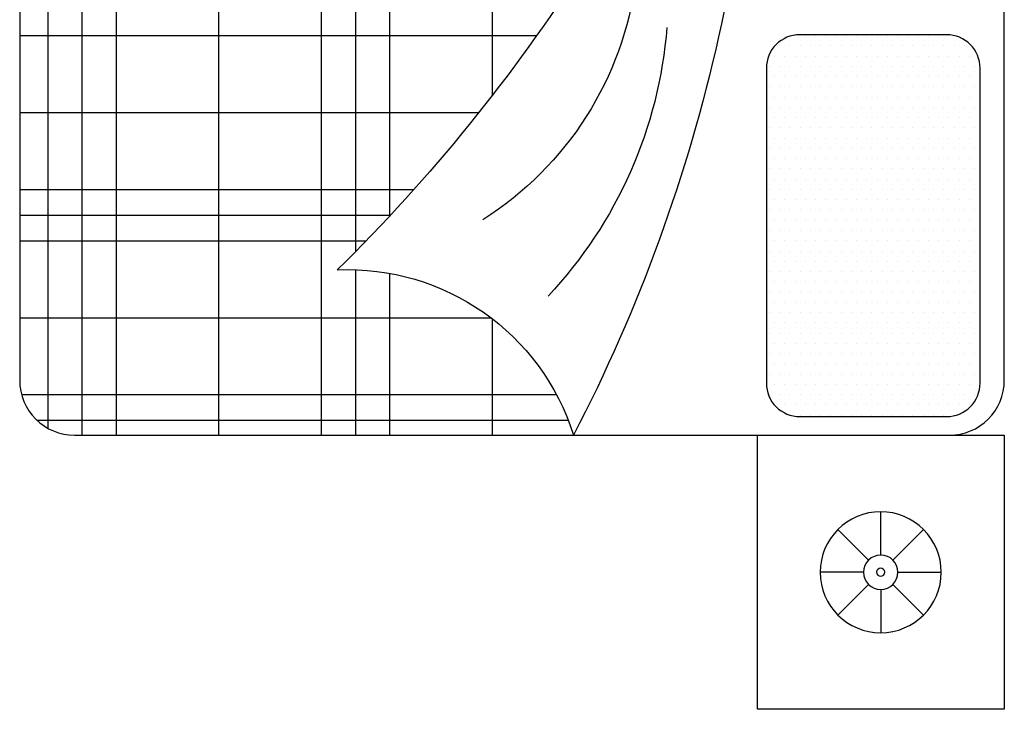
# Model space of a CAD drawing. Units: inches. Extents: x 528 to 2520, y -151 to 1354.
# Tile 11 of 41: x 814 to 869, y 1151 to 1189. Entities that reach past the tile are written whole.
import ezdxf

# ---------------------------------------------------------------- set-up
doc = ezdxf.new("R2010")
doc.units = ezdxf.units.IN
doc.header["$MEASUREMENT"] = 0
doc.layers.add('A-FURN', color=8, linetype='Continuous', lineweight=18)
doc.layers.add('BLOCK', color=6, linetype='Continuous')

# ---------------------------------------------------------------- blocks, each defined once
blk = doc.blocks.new('*X15')
at = {"color": 0}
for p, q in [((276.598, 451.25), (280.51, 451.25)), ((275.455, 450.625), (280.51, 450.625)), ((274.411, 450), (280.51, 450)), ((265.51, 448.125), (267.634, 448.125)), ((271.723, 448.125), (280.51, 448.125)), ((265.51, 446.25), (268.465, 446.25)), ((269.519, 446.25), (280.51, 446.25)), ((265.51, 445.625), (268.531, 445.625)), ((268.866, 445.625), (280.51, 445.625)), ((265.51, 445), (280.51, 445)), ((265.51, 443.125), (280.51, 443.125)), ((265.51, 441.25), (280.51, 441.25)), ((265.51, 440.625), (280.51, 440.625)), ((265.634, 440), (280.386, 440))]:
    blk.add_line(p, q, dxfattribs=at)
blk = doc.blocks.new('*X16')
at = {"color": 0}
for p, q in [((280.312, 439.886), (280.312, 452.896)), ((278.906, 439.482), (278.906, 452.338)), ((277.5, 439.482), (277.5, 451.702)), ((277.031, 439.482), (277.031, 451.471)), ((276.562, 439.482), (276.562, 451.231)), ((275.156, 439.482), (275.156, 450.451)), ((265.781, 439.797), (265.781, 449.511)), ((273.75, 439.482), (273.75, 449.576)), ((266.25, 439.517), (266.25, 449.296)), ((273.281, 439.482), (273.281, 449.261)), ((272.812, 439.482), (272.812, 448.934)), ((267.656, 439.482), (267.656, 448.095)), ((271.406, 439.482), (271.406, 447.876)), ((270, 439.482), (270, 446.689)), ((269.531, 439.482), (269.531, 446.262)), ((269.062, 439.482), (269.062, 445.817))]:
    blk.add_line(p, q, dxfattribs=at)
blk = doc.blocks.new('*X17')
at = {"color": 0}
for p, q in [((266.4375, 457.03125), (266.4375, 457.03125)), ((266.8125, 457.03125), (266.8125, 457.03125)), ((267.1875, 457.03125), (267.1875, 457.03125)), ((267.5625, 457.03125), (267.5625, 457.03125)), ((267.9375, 457.03125), (267.9375, 457.03125)), ((268.3125, 457.03125), (268.3125, 457.03125)), ((268.6875, 457.03125), (268.6875, 457.03125)), ((269.0625, 457.03125), (269.0625, 457.03125)), ((269.4375, 457.03125), (269.4375, 457.03125)), ((269.8125, 457.03125), (269.8125, 457.03125)), ((270.1875, 457.03125), (270.1875, 457.03125)), ((270.5625, 457.03125), (270.5625, 457.03125)), ((270.9375, 457.03125), (270.9375, 457.03125)), ((271.3125, 457.03125), (271.3125, 457.03125)), ((271.6875, 457.03125), (271.6875, 457.03125)), ((272.0625, 457.03125), (272.0625, 457.03125)), ((266.0625, 456.84375), (266.0625, 456.84375)), ((266.25, 456.9375), (266.25, 456.9375)), ((266.4375, 456.84375), (266.4375, 456.84375)), ((266.625, 456.9375), (266.625, 456.9375)), ((266.8125, 456.84375), (266.8125, 456.84375)), ((267, 456.9375), (267, 456.9375)), ((267.1875, 456.84375), (267.1875, 456.84375)), ((267.375, 456.9375), (267.375, 456.9375)), ((267.5625, 456.84375), (267.5625, 456.84375)), ((267.75, 456.9375), (267.75, 456.9375)), ((267.9375, 456.84375), (267.9375, 456.84375)), ((268.125, 456.9375), (268.125, 456.9375)), ((268.3125, 456.84375), (268.3125, 456.84375)), ((268.5, 456.9375), (268.5, 456.9375)), ((268.6875, 456.84375), (268.6875, 456.84375)), ((268.875, 456.9375), (268.875, 456.9375)), ((269.0625, 456.84375), (269.0625, 456.84375)), ((269.25, 456.9375), (269.25, 456.9375)), ((269.4375, 456.84375), (269.4375, 456.84375)), ((269.625, 456.9375), (269.625, 456.9375)), ((269.8125, 456.84375), (269.8125, 456.84375)), ((270, 456.9375), (270, 456.9375)), ((270.1875, 456.84375), (270.1875, 456.84375)), ((270.375, 456.9375), (270.375, 456.9375)), ((270.5625, 456.84375), (270.5625, 456.84375)), ((270.75, 456.9375), (270.75, 456.9375)), ((270.9375, 456.84375), (270.9375, 456.84375)), ((271.125, 456.9375), (271.125, 456.9375)), ((271.3125, 456.84375), (271.3125, 456.84375)), ((271.5, 456.9375), (271.5, 456.9375)), ((271.6875, 456.84375), (271.6875, 456.84375)), ((271.875, 456.9375), (271.875, 456.9375)), ((272.0625, 456.84375), (272.0625, 456.84375)), ((272.25, 456.9375), (272.25, 456.9375)), ((272.4375, 456.84375), (272.4375, 456.84375)), ((266.25, 456.75), (266.25, 456.75)), ((266.625, 456.75), (266.625, 456.75)), ((267, 456.75), (267, 456.75)), ((267.375, 456.75), (267.375, 456.75)), ((267.75, 456.75), (267.75, 456.75)), ((268.125, 456.75), (268.125, 456.75)), ((268.5, 456.75), (268.5, 456.75)), ((268.875, 456.75), (268.875, 456.75)), ((269.25, 456.75), (269.25, 456.75)), ((269.625, 456.75), (269.625, 456.75)), ((270, 456.75), (270, 456.75)), ((270.375, 456.75), (270.375, 456.75)), ((270.75, 456.75), (270.75, 456.75)), ((271.125, 456.75), (271.125, 456.75)), ((271.5, 456.75), (271.5, 456.75)), ((271.875, 456.75), (271.875, 456.75)), ((272.25, 456.75), (272.25, 456.75)), ((272.625, 456.75), (272.625, 456.75)), ((265.875, 456.5625), (265.875, 456.5625)), ((266.0625, 456.65625), (266.0625, 456.65625)), ((266.25, 456.5625), (266.25, 456.5625)), ((266.4375, 456.65625), (266.4375, 456.65625)), ((266.625, 456.5625), (266.625, 456.5625)), ((266.8125, 456.65625), (266.8125, 456.65625)), ((267, 456.5625), (267, 456.5625)), ((267.1875, 456.65625), (267.1875, 456.65625)), ((267.375, 456.5625), (267.375, 456.5625)), ((267.5625, 456.65625), (267.5625, 456.65625)), ((267.75, 456.5625), (267.75, 456.5625)), ((267.9375, 456.65625), (267.9375, 456.65625)), ((268.125, 456.5625), (268.125, 456.5625)), ((268.3125, 456.65625), (268.3125, 456.65625)), ((268.5, 456.5625), (268.5, 456.5625)), ((268.6875, 456.65625), (268.6875, 456.65625)), ((268.875, 456.5625), (268.875, 456.5625)), ((269.0625, 456.65625), (269.0625, 456.65625)), ((269.25, 456.5625), (269.25, 456.5625)), ((269.4375, 456.65625), (269.4375, 456.65625)), ((269.625, 456.5625), (269.625, 456.5625)), ((269.8125, 456.65625), (269.8125, 456.65625)), ((270, 456.5625), (270, 456.5625)), ((270.1875, 456.65625), (270.1875, 456.65625)), ((270.375, 456.5625), (270.375, 456.5625)), ((270.5625, 456.65625), (270.5625, 456.65625)), ((270.75, 456.5625), (270.75, 456.5625)), ((270.9375, 456.65625), (270.9375, 456.65625)), ((271.125, 456.5625), (271.125, 456.5625)), ((271.3125, 456.65625), (271.3125, 456.65625)), ((271.5, 456.5625), (271.5, 456.5625)), ((271.6875, 456.65625), (271.6875, 456.65625)), ((271.875, 456.5625), (271.875, 456.5625)), ((272.0625, 456.65625), (272.0625, 456.65625)), ((272.25, 456.5625), (272.25, 456.5625)), ((272.4375, 456.65625), (272.4375, 456.65625)), ((272.625, 456.5625), (272.625, 456.5625)), ((265.875, 456.375), (265.875, 456.375)), ((266.0625, 456.46875), (266.0625, 456.46875)), ((266.25, 456.375), (266.25, 456.375)), ((266.4375, 456.46875), (266.4375, 456.46875)), ((266.625, 456.375), (266.625, 456.375)), ((266.8125, 456.46875), (266.8125, 456.46875)), ((267, 456.375), (267, 456.375)), ((267.1875, 456.46875), (267.1875, 456.46875)), ((267.375, 456.375), (267.375, 456.375)), ((267.5625, 456.46875), (267.5625, 456.46875)), ((267.75, 456.375), (267.75, 456.375)), ((267.9375, 456.46875), (267.9375, 456.46875)), ((268.125, 456.375), (268.125, 456.375)), ((268.3125, 456.46875), (268.3125, 456.46875)), ((268.5, 456.375), (268.5, 456.375)), ((268.6875, 456.46875), (268.6875, 456.46875)), ((268.875, 456.375), (268.875, 456.375)), ((269.0625, 456.46875), (269.0625, 456.46875)), ((269.25, 456.375), (269.25, 456.375)), ((269.4375, 456.46875), (269.4375, 456.46875)), ((269.625, 456.375), (269.625, 456.375)), ((269.8125, 456.46875), (269.8125, 456.46875)), ((270, 456.375), (270, 456.375)), ((270.1875, 456.46875), (270.1875, 456.46875)), ((270.375, 456.375), (270.375, 456.375)), ((270.5625, 456.46875), (270.5625, 456.46875)), ((270.75, 456.375), (270.75, 456.375)), ((270.9375, 456.46875), (270.9375, 456.46875)), ((271.125, 456.375), (271.125, 456.375)), ((271.3125, 456.46875), (271.3125, 456.46875)), ((271.5, 456.375), (271.5, 456.375)), ((271.6875, 456.46875), (271.6875, 456.46875)), ((271.875, 456.375), (271.875, 456.375)), ((272.0625, 456.46875), (272.0625, 456.46875)), ((272.25, 456.375), (272.25, 456.375)), ((272.4375, 456.46875), (272.4375, 456.46875)), ((272.625, 456.375), (272.625, 456.375)), ((272.8125, 456.46875), (272.8125, 456.46875)), ((265.875, 456.1875), (265.875, 456.1875)), ((266.0625, 456.28125), (266.0625, 456.28125)), ((266.25, 456.1875), (266.25, 456.1875)), ((266.4375, 456.28125), (266.4375, 456.28125)), ((266.625, 456.1875), (266.625, 456.1875)), ((266.8125, 456.28125), (266.8125, 456.28125)), ((267, 456.1875), (267, 456.1875)), ((267.1875, 456.28125), (267.1875, 456.28125)), ((267.375, 456.1875), (267.375, 456.1875)), ((267.5625, 456.28125), (267.5625, 456.28125)), ((267.75, 456.1875), (267.75, 456.1875)), ((267.9375, 456.28125), (267.9375, 456.28125)), ((268.125, 456.1875), (268.125, 456.1875)), ((268.3125, 456.28125), (268.3125, 456.28125)), ((268.5, 456.1875), (268.5, 456.1875)), ((268.6875, 456.28125), (268.6875, 456.28125)), ((268.875, 456.1875), (268.875, 456.1875)), ((269.0625, 456.28125), (269.0625, 456.28125)), ((269.25, 456.1875), (269.25, 456.1875)), ((269.4375, 456.28125), (269.4375, 456.28125)), ((269.625, 456.1875), (269.625, 456.1875)), ((269.8125, 456.28125), (269.8125, 456.28125)), ((270, 456.1875), (270, 456.1875)), ((270.1875, 456.28125), (270.1875, 456.28125)), ((270.375, 456.1875), (270.375, 456.1875)), ((270.5625, 456.28125), (270.5625, 456.28125)), ((270.75, 456.1875), (270.75, 456.1875)), ((270.9375, 456.28125), (270.9375, 456.28125)), ((271.125, 456.1875), (271.125, 456.1875)), ((271.3125, 456.28125), (271.3125, 456.28125)), ((271.5, 456.1875), (271.5, 456.1875)), ((271.6875, 456.28125), (271.6875, 456.28125)), ((271.875, 456.1875), (271.875, 456.1875)), ((272.0625, 456.28125), (272.0625, 456.28125)), ((272.25, 456.1875), (272.25, 456.1875)), ((272.4375, 456.28125), (272.4375, 456.28125)), ((272.625, 456.1875), (272.625, 456.1875)), ((272.8125, 456.28125), (272.8125, 456.28125)), ((265.875, 456), (265.875, 456)), ((266.0625, 456.09375), (266.0625, 456.09375)), ((266.25, 456), (266.25, 456)), ((266.4375, 456.09375), (266.4375, 456.09375)), ((266.625, 456), (266.625, 456)), ((266.8125, 456.09375), (266.8125, 456.09375)), ((267, 456), (267, 456)), ((267.1875, 456.09375), (267.1875, 456.09375)), ((267.375, 456), (267.375, 456)), ((267.5625, 456.09375), (267.5625, 456.09375)), ((267.75, 456), (267.75, 456)), ((267.9375, 456.09375), (267.9375, 456.09375)), ((268.125, 456), (268.125, 456)), ((268.3125, 456.09375), (268.3125, 456.09375)), ((268.5, 456), (268.5, 456)), ((268.6875, 456.09375), (268.6875, 456.09375)), ((268.875, 456), (268.875, 456)), ((269.0625, 456.09375), (269.0625, 456.09375)), ((269.25, 456), (269.25, 456)), ((269.4375, 456.09375), (269.4375, 456.09375)), ((269.625, 456), (269.625, 456)), ((269.8125, 456.09375), (269.8125, 456.09375)), ((270, 456), (270, 456)), ((270.1875, 456.09375), (270.1875, 456.09375)), ((270.375, 456), (270.375, 456)), ((270.5625, 456.09375), (270.5625, 456.09375)), ((270.75, 456), (270.75, 456)), ((270.9375, 456.09375), (270.9375, 456.09375)), ((271.125, 456), (271.125, 456)), ((271.3125, 456.09375), (271.3125, 456.09375)), ((271.5, 456), (271.5, 456)), ((271.6875, 456.09375), (271.6875, 456.09375)), ((271.875, 456), (271.875, 456)), ((272.0625, 456.09375), (272.0625, 456.09375)), ((272.25, 456), (272.25, 456)), ((272.4375, 456.09375), (272.4375, 456.09375)), ((272.625, 456), (272.625, 456)), ((272.8125, 456.09375), (272.8125, 456.09375)), ((265.875, 455.8125), (265.875, 455.8125)), ((266.0625, 455.90625), (266.0625, 455.90625)), ((266.25, 455.8125), (266.25, 455.8125)), ((266.4375, 455.90625), (266.4375, 455.90625)), ((266.625, 455.8125), (266.625, 455.8125)), ((266.8125, 455.90625), (266.8125, 455.90625)), ((267, 455.8125), (267, 455.8125)), ((267.1875, 455.90625), (267.1875, 455.90625)), ((267.375, 455.8125), (267.375, 455.8125)), ((267.5625, 455.90625), (267.5625, 455.90625)), ((267.75, 455.8125), (267.75, 455.8125)), ((267.9375, 455.90625), (267.9375, 455.90625)), ((268.125, 455.8125), (268.125, 455.8125)), ((268.3125, 455.90625), (268.3125, 455.90625)), ((268.5, 455.8125), (268.5, 455.8125)), ((268.6875, 455.90625), (268.6875, 455.90625)), ((268.875, 455.8125), (268.875, 455.8125)), ((269.0625, 455.90625), (269.0625, 455.90625)), ((269.25, 455.8125), (269.25, 455.8125)), ((269.4375, 455.90625), (269.4375, 455.90625)), ((269.625, 455.8125), (269.625, 455.8125)), ((269.8125, 455.90625), (269.8125, 455.90625)), ((270, 455.8125), (270, 455.8125)), ((270.1875, 455.90625), (270.1875, 455.90625)), ((270.375, 455.8125), (270.375, 455.8125)), ((270.5625, 455.90625), (270.5625, 455.90625)), ((270.75, 455.8125), (270.75, 455.8125)), ((270.9375, 455.90625), (270.9375, 455.90625)), ((271.125, 455.8125), (271.125, 455.8125)), ((271.3125, 455.90625), (271.3125, 455.90625)), ((271.5, 455.8125), (271.5, 455.8125)), ((271.6875, 455.90625), (271.6875, 455.90625)), ((271.875, 455.8125), (271.875, 455.8125)), ((272.0625, 455.90625), (272.0625, 455.90625)), ((272.25, 455.8125), (272.25, 455.8125)), ((272.4375, 455.90625), (272.4375, 455.90625)), ((272.625, 455.8125), (272.625, 455.8125)), ((272.8125, 455.90625), (272.8125, 455.90625)), ((265.875, 455.625), (265.875, 455.625)), ((266.0625, 455.71875), (266.0625, 455.71875)), ((266.25, 455.625), (266.25, 455.625)), ((266.4375, 455.71875), (266.4375, 455.71875)), ((266.625, 455.625), (266.625, 455.625)), ((266.8125, 455.71875), (266.8125, 455.71875)), ((267, 455.625), (267, 455.625)), ((267.1875, 455.71875), (267.1875, 455.71875)), ((267.375, 455.625), (267.375, 455.625)), ((267.5625, 455.71875), (267.5625, 455.71875)), ((267.75, 455.625), (267.75, 455.625)), ((267.9375, 455.71875), (267.9375, 455.71875)), ((268.125, 455.625), (268.125, 455.625)), ((268.3125, 455.71875), (268.3125, 455.71875)), ((268.5, 455.625), (268.5, 455.625)), ((268.6875, 455.71875), (268.6875, 455.71875)), ((268.875, 455.625), (268.875, 455.625)), ((269.0625, 455.71875), (269.0625, 455.71875)), ((269.25, 455.625), (269.25, 455.625)), ((269.4375, 455.71875), (269.4375, 455.71875)), ((269.625, 455.625), (269.625, 455.625)), ((269.8125, 455.71875), (269.8125, 455.71875)), ((270, 455.625), (270, 455.625)), ((270.1875, 455.71875), (270.1875, 455.71875)), ((270.375, 455.625), (270.375, 455.625)), ((270.5625, 455.71875), (270.5625, 455.71875)), ((270.75, 455.625), (270.75, 455.625)), ((270.9375, 455.71875), (270.9375, 455.71875)), ((271.125, 455.625), (271.125, 455.625)), ((271.3125, 455.71875), (271.3125, 455.71875)), ((271.5, 455.625), (271.5, 455.625)), ((271.6875, 455.71875), (271.6875, 455.71875)), ((271.875, 455.625), (271.875, 455.625)), ((272.0625, 455.71875), (272.0625, 455.71875)), ((272.25, 455.625), (272.25, 455.625)), ((272.4375, 455.71875), (272.4375, 455.71875)), ((272.625, 455.625), (272.625, 455.625)), ((272.8125, 455.71875), (272.8125, 455.71875)), ((265.875, 455.4375), (265.875, 455.4375)), ((266.0625, 455.53125), (266.0625, 455.53125)), ((266.25, 455.4375), (266.25, 455.4375)), ((266.4375, 455.53125), (266.4375, 455.53125)), ((266.625, 455.4375), (266.625, 455.4375)), ((266.8125, 455.53125), (266.8125, 455.53125)), ((267, 455.4375), (267, 455.4375)), ((267.1875, 455.53125), (267.1875, 455.53125)), ((267.375, 455.4375), (267.375, 455.4375)), ((267.5625, 455.53125), (267.5625, 455.53125)), ((267.75, 455.4375), (267.75, 455.4375)), ((267.9375, 455.53125), (267.9375, 455.53125)), ((268.125, 455.4375), (268.125, 455.4375)), ((268.3125, 455.53125), (268.3125, 455.53125)), ((268.5, 455.4375), (268.5, 455.4375)), ((268.6875, 455.53125), (268.6875, 455.53125)), ((268.875, 455.4375), (268.875, 455.4375)), ((269.0625, 455.53125), (269.0625, 455.53125)), ((269.25, 455.4375), (269.25, 455.4375)), ((269.4375, 455.53125), (269.4375, 455.53125)), ((269.625, 455.4375), (269.625, 455.4375)), ((269.8125, 455.53125), (269.8125, 455.53125)), ((270, 455.4375), (270, 455.4375)), ((270.1875, 455.53125), (270.1875, 455.53125)), ((270.375, 455.4375), (270.375, 455.4375)), ((270.5625, 455.53125), (270.5625, 455.53125)), ((270.75, 455.4375), (270.75, 455.4375)), ((270.9375, 455.53125), (270.9375, 455.53125)), ((271.125, 455.4375), (271.125, 455.4375)), ((271.3125, 455.53125), (271.3125, 455.53125)), ((271.5, 455.4375), (271.5, 455.4375)), ((271.6875, 455.53125), (271.6875, 455.53125)), ((271.875, 455.4375), (271.875, 455.4375)), ((272.0625, 455.53125), (272.0625, 455.53125)), ((272.25, 455.4375), (272.25, 455.4375)), ((272.4375, 455.53125), (272.4375, 455.53125)), ((272.625, 455.4375), (272.625, 455.4375)), ((272.8125, 455.53125), (272.8125, 455.53125)), ((265.875, 455.25), (265.875, 455.25)), ((266.0625, 455.34375), (266.0625, 455.34375)), ((266.25, 455.25), (266.25, 455.25)), ((266.4375, 455.34375), (266.4375, 455.34375)), ((266.625, 455.25), (266.625, 455.25)), ((266.8125, 455.34375), (266.8125, 455.34375)), ((267, 455.25), (267, 455.25)), ((267.1875, 455.34375), (267.1875, 455.34375)), ((267.375, 455.25), (267.375, 455.25)), ((267.5625, 455.34375), (267.5625, 455.34375)), ((267.75, 455.25), (267.75, 455.25)), ((267.9375, 455.34375), (267.9375, 455.34375)), ((268.125, 455.25), (268.125, 455.25)), ((268.3125, 455.34375), (268.3125, 455.34375)), ((268.5, 455.25), (268.5, 455.25)), ((268.6875, 455.34375), (268.6875, 455.34375)), ((268.875, 455.25), (268.875, 455.25)), ((269.0625, 455.34375), (269.0625, 455.34375)), ((269.25, 455.25), (269.25, 455.25)), ((269.4375, 455.34375), (269.4375, 455.34375)), ((269.625, 455.25), (269.625, 455.25)), ((269.8125, 455.34375), (269.8125, 455.34375)), ((270, 455.25), (270, 455.25)), ((270.1875, 455.34375), (270.1875, 455.34375)), ((270.375, 455.25), (270.375, 455.25)), ((270.5625, 455.34375), (270.5625, 455.34375)), ((270.75, 455.25), (270.75, 455.25)), ((270.9375, 455.34375), (270.9375, 455.34375)), ((271.125, 455.25), (271.125, 455.25)), ((271.3125, 455.34375), (271.3125, 455.34375)), ((271.5, 455.25), (271.5, 455.25)), ((271.6875, 455.34375), (271.6875, 455.34375)), ((271.875, 455.25), (271.875, 455.25)), ((272.0625, 455.34375), (272.0625, 455.34375)), ((272.25, 455.25), (272.25, 455.25)), ((272.4375, 455.34375), (272.4375, 455.34375)), ((272.625, 455.25), (272.625, 455.25)), ((272.8125, 455.34375), (272.8125, 455.34375)), ((265.875, 455.0625), (265.875, 455.0625)), ((266.0625, 455.15625), (266.0625, 455.15625)), ((266.25, 455.0625), (266.25, 455.0625)), ((266.4375, 455.15625), (266.4375, 455.15625)), ((266.625, 455.0625), (266.625, 455.0625)), ((266.8125, 455.15625), (266.8125, 455.15625)), ((267, 455.0625), (267, 455.0625)), ((267.1875, 455.15625), (267.1875, 455.15625)), ((267.375, 455.0625), (267.375, 455.0625)), ((267.5625, 455.15625), (267.5625, 455.15625)), ((267.75, 455.0625), (267.75, 455.0625)), ((267.9375, 455.15625), (267.9375, 455.15625)), ((268.125, 455.0625), (268.125, 455.0625)), ((268.3125, 455.15625), (268.3125, 455.15625)), ((268.5, 455.0625), (268.5, 455.0625)), ((268.6875, 455.15625), (268.6875, 455.15625)), ((268.875, 455.0625), (268.875, 455.0625)), ((269.0625, 455.15625), (269.0625, 455.15625)), ((269.25, 455.0625), (269.25, 455.0625)), ((269.4375, 455.15625), (269.4375, 455.15625)), ((269.625, 455.0625), (269.625, 455.0625)), ((269.8125, 455.15625), (269.8125, 455.15625)), ((270, 455.0625), (270, 455.0625)), ((270.1875, 455.15625), (270.1875, 455.15625)), ((270.375, 455.0625), (270.375, 455.0625)), ((270.5625, 455.15625), (270.5625, 455.15625)), ((270.75, 455.0625), (270.75, 455.0625)), ((270.9375, 455.15625), (270.9375, 455.15625)), ((271.125, 455.0625), (271.125, 455.0625)), ((271.3125, 455.15625), (271.3125, 455.15625)), ((271.5, 455.0625), (271.5, 455.0625)), ((271.6875, 455.15625), (271.6875, 455.15625)), ((271.875, 455.0625), (271.875, 455.0625)), ((272.0625, 455.15625), (272.0625, 455.15625)), ((272.25, 455.0625), (272.25, 455.0625)), ((272.4375, 455.15625), (272.4375, 455.15625)), ((272.625, 455.0625), (272.625, 455.0625)), ((272.8125, 455.15625), (272.8125, 455.15625)), ((265.875, 454.875), (265.875, 454.875)), ((266.0625, 454.96875), (266.0625, 454.96875)), ((266.25, 454.875), (266.25, 454.875)), ((266.4375, 454.96875), (266.4375, 454.96875)), ((266.625, 454.875), (266.625, 454.875)), ((266.8125, 454.96875), (266.8125, 454.96875)), ((267, 454.875), (267, 454.875)), ((267.1875, 454.96875), (267.1875, 454.96875)), ((267.375, 454.875), (267.375, 454.875)), ((267.5625, 454.96875), (267.5625, 454.96875)), ((267.75, 454.875), (267.75, 454.875)), ((267.9375, 454.96875), (267.9375, 454.96875)), ((268.125, 454.875), (268.125, 454.875)), ((268.3125, 454.96875), (268.3125, 454.96875)), ((268.5, 454.875), (268.5, 454.875)), ((268.6875, 454.96875), (268.6875, 454.96875)), ((268.875, 454.875), (268.875, 454.875)), ((269.0625, 454.96875), (269.0625, 454.96875)), ((269.25, 454.875), (269.25, 454.875)), ((269.4375, 454.96875), (269.4375, 454.96875)), ((269.625, 454.875), (269.625, 454.875)), ((269.8125, 454.96875), (269.8125, 454.96875)), ((270, 454.875), (270, 454.875)), ((270.1875, 454.96875), (270.1875, 454.96875)), ((270.375, 454.875), (270.375, 454.875)), ((270.5625, 454.96875), (270.5625, 454.96875)), ((270.75, 454.875), (270.75, 454.875)), ((270.9375, 454.96875), (270.9375, 454.96875)), ((271.125, 454.875), (271.125, 454.875)), ((271.3125, 454.96875), (271.3125, 454.96875)), ((271.5, 454.875), (271.5, 454.875)), ((271.6875, 454.96875), (271.6875, 454.96875)), ((271.875, 454.875), (271.875, 454.875)), ((272.0625, 454.96875), (272.0625, 454.96875)), ((272.25, 454.875), (272.25, 454.875)), ((272.4375, 454.96875), (272.4375, 454.96875)), ((272.625, 454.875), (272.625, 454.875)), ((272.8125, 454.96875), (272.8125, 454.96875)), ((265.875, 454.6875), (265.875, 454.6875)), ((266.0625, 454.78125), (266.0625, 454.78125)), ((266.25, 454.6875), (266.25, 454.6875)), ((266.4375, 454.78125), (266.4375, 454.78125)), ((266.625, 454.6875), (266.625, 454.6875)), ((266.8125, 454.78125), (266.8125, 454.78125)), ((267, 454.6875), (267, 454.6875)), ((267.1875, 454.78125), (267.1875, 454.78125)), ((267.375, 454.6875), (267.375, 454.6875)), ((267.5625, 454.78125), (267.5625, 454.78125)), ((267.75, 454.6875), (267.75, 454.6875)), ((267.9375, 454.78125), (267.9375, 454.78125)), ((268.125, 454.6875), (268.125, 454.6875)), ((268.3125, 454.78125), (268.3125, 454.78125)), ((268.5, 454.6875), (268.5, 454.6875)), ((268.6875, 454.78125), (268.6875, 454.78125)), ((268.875, 454.6875), (268.875, 454.6875)), ((269.0625, 454.78125), (269.0625, 454.78125)), ((269.25, 454.6875), (269.25, 454.6875)), ((269.4375, 454.78125), (269.4375, 454.78125)), ((269.625, 454.6875), (269.625, 454.6875)), ((269.8125, 454.78125), (269.8125, 454.78125)), ((270, 454.6875), (270, 454.6875)), ((270.1875, 454.78125), (270.1875, 454.78125)), ((270.375, 454.6875), (270.375, 454.6875)), ((270.5625, 454.78125), (270.5625, 454.78125)), ((270.75, 454.6875), (270.75, 454.6875)), ((270.9375, 454.78125), (270.9375, 454.78125)), ((271.125, 454.6875), (271.125, 454.6875)), ((271.3125, 454.78125), (271.3125, 454.78125)), ((271.5, 454.6875), (271.5, 454.6875)), ((271.6875, 454.78125), (271.6875, 454.78125)), ((271.875, 454.6875), (271.875, 454.6875)), ((272.0625, 454.78125), (272.0625, 454.78125)), ((272.25, 454.6875), (272.25, 454.6875)), ((272.4375, 454.78125), (272.4375, 454.78125)), ((272.625, 454.6875), (272.625, 454.6875)), ((272.8125, 454.78125), (272.8125, 454.78125)), ((266.0625, 454.59375), (266.0625, 454.59375)), ((266.4375, 454.59375), (266.4375, 454.59375)), ((266.8125, 454.59375), (266.8125, 454.59375)), ((267.1875, 454.59375), (267.1875, 454.59375)), ((267.5625, 454.59375), (267.5625, 454.59375)), ((267.9375, 454.59375), (267.9375, 454.59375)), ((268.3125, 454.59375), (268.3125, 454.59375)), ((268.6875, 454.59375), (268.6875, 454.59375)), ((269.0625, 454.59375), (269.0625, 454.59375)), ((269.4375, 454.59375), (269.4375, 454.59375)), ((269.8125, 454.59375), (269.8125, 454.59375)), ((270.1875, 454.59375), (270.1875, 454.59375)), ((270.5625, 454.59375), (270.5625, 454.59375)), ((270.9375, 454.59375), (270.9375, 454.59375)), ((271.3125, 454.59375), (271.3125, 454.59375)), ((271.6875, 454.59375), (271.6875, 454.59375)), ((272.0625, 454.59375), (272.0625, 454.59375)), ((272.4375, 454.59375), (272.4375, 454.59375)), ((272.8125, 454.59375), (272.8125, 454.59375)), ((265.875, 454.5), (265.875, 454.5)), ((266.0625, 454.40625), (266.0625, 454.40625)), ((266.25, 454.5), (266.25, 454.5)), ((266.4375, 454.40625), (266.4375, 454.40625)), ((266.625, 454.5), (266.625, 454.5)), ((266.8125, 454.40625), (266.8125, 454.40625)), ((267, 454.5), (267, 454.5)), ((267.1875, 454.40625), (267.1875, 454.40625)), ((267.375, 454.5), (267.375, 454.5)), ((267.5625, 454.40625), (267.5625, 454.40625)), ((267.75, 454.5), (267.75, 454.5)), ((267.9375, 454.40625), (267.9375, 454.40625)), ((268.125, 454.5), (268.125, 454.5)), ((268.3125, 454.40625), (268.3125, 454.40625)), ((268.5, 454.5), (268.5, 454.5)), ((268.6875, 454.40625), (268.6875, 454.40625)), ((268.875, 454.5), (268.875, 454.5)), ((269.0625, 454.40625), (269.0625, 454.40625)), ((269.25, 454.5), (269.25, 454.5)), ((269.4375, 454.40625), (269.4375, 454.40625)), ((269.625, 454.5), (269.625, 454.5)), ((269.8125, 454.40625), (269.8125, 454.40625)), ((270, 454.5), (270, 454.5)), ((270.1875, 454.40625), (270.1875, 454.40625)), ((270.375, 454.5), (270.375, 454.5)), ((270.5625, 454.40625), (270.5625, 454.40625)), ((270.75, 454.5), (270.75, 454.5)), ((270.9375, 454.40625), (270.9375, 454.40625)), ((271.125, 454.5), (271.125, 454.5)), ((271.3125, 454.40625), (271.3125, 454.40625)), ((271.5, 454.5), (271.5, 454.5)), ((271.6875, 454.40625), (271.6875, 454.40625)), ((271.875, 454.5), (271.875, 454.5)), ((272.0625, 454.40625), (272.0625, 454.40625)), ((272.25, 454.5), (272.25, 454.5)), ((272.4375, 454.40625), (272.4375, 454.40625)), ((272.625, 454.5), (272.625, 454.5)), ((272.8125, 454.40625), (272.8125, 454.40625)), ((265.875, 454.3125), (265.875, 454.3125)), ((266.0625, 454.21875), (266.0625, 454.21875)), ((266.25, 454.3125), (266.25, 454.3125)), ((266.4375, 454.21875), (266.4375, 454.21875)), ((266.625, 454.3125), (266.625, 454.3125)), ((266.8125, 454.21875), (266.8125, 454.21875)), ((267, 454.3125), (267, 454.3125)), ((267.1875, 454.21875), (267.1875, 454.21875)), ((267.375, 454.3125), (267.375, 454.3125)), ((267.5625, 454.21875), (267.5625, 454.21875)), ((267.75, 454.3125), (267.75, 454.3125)), ((267.9375, 454.21875), (267.9375, 454.21875)), ((268.125, 454.3125), (268.125, 454.3125)), ((268.3125, 454.21875), (268.3125, 454.21875)), ((268.5, 454.3125), (268.5, 454.3125)), ((268.6875, 454.21875), (268.6875, 454.21875)), ((268.875, 454.3125), (268.875, 454.3125)), ((269.0625, 454.21875), (269.0625, 454.21875)), ((269.25, 454.3125), (269.25, 454.3125)), ((269.4375, 454.21875), (269.4375, 454.21875)), ((269.625, 454.3125), (269.625, 454.3125)), ((269.8125, 454.21875), (269.8125, 454.21875)), ((270, 454.3125), (270, 454.3125)), ((270.1875, 454.21875), (270.1875, 454.21875)), ((270.375, 454.3125), (270.375, 454.3125)), ((270.5625, 454.21875), (270.5625, 454.21875)), ((270.75, 454.3125), (270.75, 454.3125)), ((270.9375, 454.21875), (270.9375, 454.21875)), ((271.125, 454.3125), (271.125, 454.3125)), ((271.3125, 454.21875), (271.3125, 454.21875)), ((271.5, 454.3125), (271.5, 454.3125)), ((271.6875, 454.21875), (271.6875, 454.21875)), ((271.875, 454.3125), (271.875, 454.3125)), ((272.0625, 454.21875), (272.0625, 454.21875)), ((272.25, 454.3125), (272.25, 454.3125)), ((272.4375, 454.21875), (272.4375, 454.21875)), ((272.625, 454.3125), (272.625, 454.3125)), ((272.8125, 454.21875), (272.8125, 454.21875)), ((265.875, 454.125), (265.875, 454.125)), ((266.0625, 454.03125), (266.0625, 454.03125)), ((266.25, 454.125), (266.25, 454.125)), ((266.4375, 454.03125), (266.4375, 454.03125)), ((266.625, 454.125), (266.625, 454.125)), ((266.8125, 454.03125), (266.8125, 454.03125)), ((267, 454.125), (267, 454.125)), ((267.1875, 454.03125), (267.1875, 454.03125)), ((267.375, 454.125), (267.375, 454.125)), ((267.5625, 454.03125), (267.5625, 454.03125)), ((267.75, 454.125), (267.75, 454.125)), ((267.9375, 454.03125), (267.9375, 454.03125)), ((268.125, 454.125), (268.125, 454.125)), ((268.3125, 454.03125), (268.3125, 454.03125)), ((268.5, 454.125), (268.5, 454.125)), ((268.6875, 454.03125), (268.6875, 454.03125)), ((268.875, 454.125), (268.875, 454.125)), ((269.0625, 454.03125), (269.0625, 454.03125)), ((269.25, 454.125), (269.25, 454.125)), ((269.4375, 454.03125), (269.4375, 454.03125)), ((269.625, 454.125), (269.625, 454.125)), ((269.8125, 454.03125), (269.8125, 454.03125)), ((270, 454.125), (270, 454.125)), ((270.1875, 454.03125), (270.1875, 454.03125)), ((270.375, 454.125), (270.375, 454.125)), ((270.5625, 454.03125), (270.5625, 454.03125)), ((270.75, 454.125), (270.75, 454.125)), ((270.9375, 454.03125), (270.9375, 454.03125)), ((271.125, 454.125), (271.125, 454.125)), ((271.3125, 454.03125), (271.3125, 454.03125)), ((271.5, 454.125), (271.5, 454.125)), ((271.6875, 454.03125), (271.6875, 454.03125)), ((271.875, 454.125), (271.875, 454.125)), ((272.0625, 454.03125), (272.0625, 454.03125)), ((272.25, 454.125), (272.25, 454.125)), ((272.4375, 454.03125), (272.4375, 454.03125)), ((272.625, 454.125), (272.625, 454.125)), ((272.8125, 454.03125), (272.8125, 454.03125)), ((265.875, 453.9375), (265.875, 453.9375)), ((266.0625, 453.84375), (266.0625, 453.84375)), ((266.25, 453.9375), (266.25, 453.9375)), ((266.4375, 453.84375), (266.4375, 453.84375)), ((266.625, 453.9375), (266.625, 453.9375)), ((266.8125, 453.84375), (266.8125, 453.84375)), ((267, 453.9375), (267, 453.9375)), ((267.1875, 453.84375), (267.1875, 453.84375)), ((267.375, 453.9375), (267.375, 453.9375)), ((267.5625, 453.84375), (267.5625, 453.84375)), ((267.75, 453.9375), (267.75, 453.9375)), ((267.9375, 453.84375), (267.9375, 453.84375)), ((268.125, 453.9375), (268.125, 453.9375)), ((268.3125, 453.84375), (268.3125, 453.84375)), ((268.5, 453.9375), (268.5, 453.9375)), ((268.6875, 453.84375), (268.6875, 453.84375)), ((268.875, 453.9375), (268.875, 453.9375)), ((269.0625, 453.84375), (269.0625, 453.84375)), ((269.25, 453.9375), (269.25, 453.9375)), ((269.4375, 453.84375), (269.4375, 453.84375)), ((269.625, 453.9375), (269.625, 453.9375)), ((269.8125, 453.84375), (269.8125, 453.84375)), ((270, 453.9375), (270, 453.9375)), ((270.1875, 453.84375), (270.1875, 453.84375)), ((270.375, 453.9375), (270.375, 453.9375)), ((270.5625, 453.84375), (270.5625, 453.84375)), ((270.75, 453.9375), (270.75, 453.9375)), ((270.9375, 453.84375), (270.9375, 453.84375)), ((271.125, 453.9375), (271.125, 453.9375)), ((271.3125, 453.84375), (271.3125, 453.84375)), ((271.5, 453.9375), (271.5, 453.9375)), ((271.6875, 453.84375), (271.6875, 453.84375)), ((271.875, 453.9375), (271.875, 453.9375)), ((272.0625, 453.84375), (272.0625, 453.84375)), ((272.25, 453.9375), (272.25, 453.9375)), ((272.4375, 453.84375), (272.4375, 453.84375)), ((272.625, 453.9375), (272.625, 453.9375)), ((272.8125, 453.84375), (272.8125, 453.84375)), ((265.875, 453.75), (265.875, 453.75)), ((266.0625, 453.65625), (266.0625, 453.65625)), ((266.25, 453.75), (266.25, 453.75)), ((266.4375, 453.65625), (266.4375, 453.65625)), ((266.625, 453.75), (266.625, 453.75)), ((266.8125, 453.65625), (266.8125, 453.65625)), ((267, 453.75), (267, 453.75)), ((267.1875, 453.65625), (267.1875, 453.65625)), ((267.375, 453.75), (267.375, 453.75)), ((267.5625, 453.65625), (267.5625, 453.65625)), ((267.75, 453.75), (267.75, 453.75)), ((267.9375, 453.65625), (267.9375, 453.65625)), ((268.125, 453.75), (268.125, 453.75)), ((268.3125, 453.65625), (268.3125, 453.65625)), ((268.5, 453.75), (268.5, 453.75)), ((268.6875, 453.65625), (268.6875, 453.65625)), ((268.875, 453.75), (268.875, 453.75)), ((269.0625, 453.65625), (269.0625, 453.65625)), ((269.25, 453.75), (269.25, 453.75)), ((269.4375, 453.65625), (269.4375, 453.65625)), ((269.625, 453.75), (269.625, 453.75)), ((269.8125, 453.65625), (269.8125, 453.65625)), ((270, 453.75), (270, 453.75)), ((270.1875, 453.65625), (270.1875, 453.65625)), ((270.375, 453.75), (270.375, 453.75)), ((270.5625, 453.65625), (270.5625, 453.65625)), ((270.75, 453.75), (270.75, 453.75)), ((270.9375, 453.65625), (270.9375, 453.65625)), ((271.125, 453.75), (271.125, 453.75)), ((271.3125, 453.65625), (271.3125, 453.65625)), ((271.5, 453.75), (271.5, 453.75)), ((271.6875, 453.65625), (271.6875, 453.65625)), ((271.875, 453.75), (271.875, 453.75)), ((272.0625, 453.65625), (272.0625, 453.65625)), ((272.25, 453.75), (272.25, 453.75)), ((272.4375, 453.65625), (272.4375, 453.65625)), ((272.625, 453.75), (272.625, 453.75)), ((272.8125, 453.65625), (272.8125, 453.65625)), ((266.0625, 453.46875), (266.0625, 453.46875)), ((266.25, 453.5625), (266.25, 453.5625)), ((266.4375, 453.46875), (266.4375, 453.46875)), ((266.625, 453.5625), (266.625, 453.5625)), ((266.8125, 453.46875), (266.8125, 453.46875)), ((267, 453.5625), (267, 453.5625)), ((267.1875, 453.46875), (267.1875, 453.46875)), ((267.375, 453.5625), (267.375, 453.5625)), ((267.5625, 453.46875), (267.5625, 453.46875)), ((267.75, 453.5625), (267.75, 453.5625)), ((267.9375, 453.46875), (267.9375, 453.46875)), ((268.125, 453.5625), (268.125, 453.5625)), ((268.3125, 453.46875), (268.3125, 453.46875)), ((268.5, 453.5625), (268.5, 453.5625)), ((268.6875, 453.46875), (268.6875, 453.46875)), ((268.875, 453.5625), (268.875, 453.5625)), ((269.0625, 453.46875), (269.0625, 453.46875)), ((269.25, 453.5625), (269.25, 453.5625)), ((269.4375, 453.46875), (269.4375, 453.46875)), ((269.625, 453.5625), (269.625, 453.5625)), ((269.8125, 453.46875), (269.8125, 453.46875)), ((270, 453.5625), (270, 453.5625)), ((270.1875, 453.46875), (270.1875, 453.46875)), ((270.375, 453.5625), (270.375, 453.5625)), ((270.5625, 453.46875), (270.5625, 453.46875)), ((270.75, 453.5625), (270.75, 453.5625)), ((270.9375, 453.46875), (270.9375, 453.46875)), ((271.125, 453.5625), (271.125, 453.5625)), ((271.3125, 453.46875), (271.3125, 453.46875)), ((271.5, 453.5625), (271.5, 453.5625)), ((271.6875, 453.46875), (271.6875, 453.46875)), ((271.875, 453.5625), (271.875, 453.5625)), ((272.0625, 453.46875), (272.0625, 453.46875)), ((272.25, 453.5625), (272.25, 453.5625)), ((272.4375, 453.46875), (272.4375, 453.46875)), ((272.625, 453.5625), (272.625, 453.5625)), ((266.0625, 453.28125), (266.0625, 453.28125)), ((266.25, 453.375), (266.25, 453.375)), ((266.4375, 453.28125), (266.4375, 453.28125)), ((266.625, 453.375), (266.625, 453.375)), ((266.8125, 453.28125), (266.8125, 453.28125)), ((267, 453.375), (267, 453.375)), ((267.1875, 453.28125), (267.1875, 453.28125)), ((267.375, 453.375), (267.375, 453.375)), ((267.5625, 453.28125), (267.5625, 453.28125)), ((267.75, 453.375), (267.75, 453.375)), ((267.9375, 453.28125), (267.9375, 453.28125)), ((268.125, 453.375), (268.125, 453.375)), ((268.3125, 453.28125), (268.3125, 453.28125)), ((268.5, 453.375), (268.5, 453.375)), ((268.6875, 453.28125), (268.6875, 453.28125)), ((268.875, 453.375), (268.875, 453.375)), ((269.0625, 453.28125), (269.0625, 453.28125)), ((269.25, 453.375), (269.25, 453.375)), ((269.4375, 453.28125), (269.4375, 453.28125)), ((269.625, 453.375), (269.625, 453.375)), ((269.8125, 453.28125), (269.8125, 453.28125)), ((270, 453.375), (270, 453.375)), ((270.1875, 453.28125), (270.1875, 453.28125)), ((270.375, 453.375), (270.375, 453.375)), ((270.5625, 453.28125), (270.5625, 453.28125)), ((270.75, 453.375), (270.75, 453.375)), ((270.9375, 453.28125), (270.9375, 453.28125)), ((271.125, 453.375), (271.125, 453.375)), ((271.3125, 453.28125), (271.3125, 453.28125)), ((271.5, 453.375), (271.5, 453.375)), ((271.6875, 453.28125), (271.6875, 453.28125)), ((271.875, 453.375), (271.875, 453.375)), ((272.0625, 453.28125), (272.0625, 453.28125)), ((272.25, 453.375), (272.25, 453.375)), ((272.4375, 453.28125), (272.4375, 453.28125)), ((272.625, 453.375), (272.625, 453.375)), ((266.25, 453.1875), (266.25, 453.1875)), ((266.625, 453.1875), (266.625, 453.1875)), ((267, 453.1875), (267, 453.1875)), ((267.375, 453.1875), (267.375, 453.1875)), ((267.75, 453.1875), (267.75, 453.1875)), ((268.125, 453.1875), (268.125, 453.1875)), ((268.5, 453.1875), (268.5, 453.1875)), ((268.875, 453.1875), (268.875, 453.1875)), ((269.25, 453.1875), (269.25, 453.1875)), ((269.625, 453.1875), (269.625, 453.1875)), ((270, 453.1875), (270, 453.1875)), ((270.375, 453.1875), (270.375, 453.1875)), ((270.75, 453.1875), (270.75, 453.1875)), ((271.125, 453.1875), (271.125, 453.1875)), ((271.5, 453.1875), (271.5, 453.1875)), ((271.875, 453.1875), (271.875, 453.1875)), ((272.25, 453.1875), (272.25, 453.1875))]:
    blk.add_line(p, q, dxfattribs=at)
blk = doc.blocks.new('A$C52E67D0D')
at = {"layer": 'BLOCK'}
for p, q in [((250.5, 1605.5), (250.5, 1684.7)), ((228.3, 1596.3), (172.3, 1652.3)), ((272.7, 1596.3), (328.7, 1652.3)), ((219.1, 1574.1), (139.9, 1574.1)), ((281.9, 1574.1), (361.1, 1574.1)), ((228.3, 1551.9), (172.3, 1495.9)), ((272.7, 1551.9), (328.7, 1495.9)), ((250.5, 1542.8), (250.5, 1463.5))]:
    blk.add_line(p, q, dxfattribs=at)
for points in [[(1901, 0), (601, 0, -0.414214), (501, 100), (501, 1700, -0.414214), (601, 1800), (1901, 1800, -0.414214), (2001, 1700), (2001, 100, -0.414214)], [(1171.8, 1365.1), (595.8, 1365.1, -0.414214), (535, 1425.9), (535, 1694.8, -0.414214), (595.8, 1755.7), (1171.8, 1755.7, -0.414214), (1232.6, 1694.8), (1232.6, 1425.9, -0.414214)]]:
    blk.add_lwpolyline(points, format="xyb", close=True, dxfattribs=at)
blk.add_lwpolyline([(501, 1348.6), (501, 1799.6), (0, 1799.6), (0, 1348.6)], close=True, dxfattribs=at)
for radius in [110.6, 31.4, 7.46]:
    blk.add_circle((250.5, 1574.1), radius, dxfattribs=at)
for centre, radius, start, end in [((1888.6, -1664.5), 3015.3, 87.8642, 117.4001), ((3101, -1685.8), 3227.7, 109.926, 135.3977), ((1308.8, 377.9), 807.6, 94.4436, 133.2788), ((1410.8, 520.2), 610.8, 97.2157, 147.6656), ((371.4, 600.4), 432, 357.3792, 72.5379)]:
    blk.add_arc(centre, radius, start, end, dxfattribs=at)
at = {"layer": 'BLOCK', "xscale": 100, "yscale": 100, "zscale": 100}
for name in ['*X17', '*X16', '*X15']:
    blk.add_blockref(name, (-26050, -43948.2), dxfattribs=at)

msp = doc.modelspace()

# ---------------------------------------------------------------- block references
at = {"layer": 'A-FURN', "xscale": -0.0306954436450662, "yscale": 0.0306954436450662, "zscale": 0.0306954436450662, "rotation": 270}
msp.add_blockref('A$C52E67D0D', (813.801, 1150.631), dxfattribs=at)

doc.saveas('drawing.dxf')
